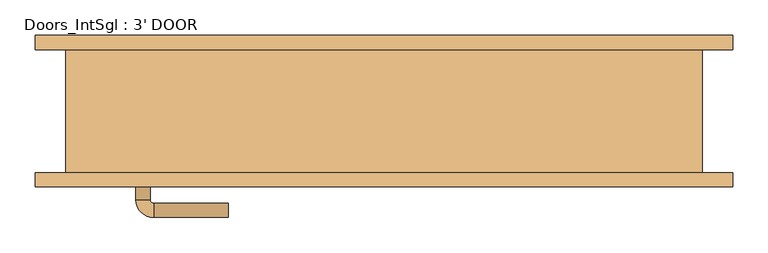
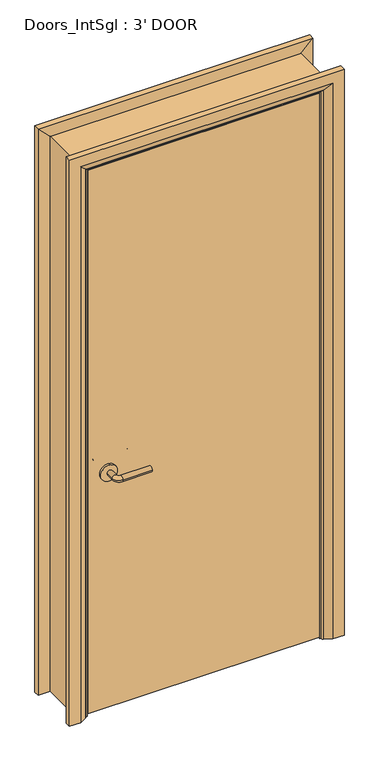
"""IFC4 building model written with IfcOpenShell, lengths in millimetres: door geometry, Doors_IntSgl : 3' DOOR."""

from ifc_helpers import new_model, si_unit, point, frame, frame_2d, origin, place, context, project, spatial, polyline, circle_curve, ellipse_curve, trimmed, segment, composite_curve, outline, extrude, faceted_brep, source, transform, mapped, element, save
from ifc_brep_helpers import plane_surface, cylinder_surface, revolved_surface, advanced_brep


def doors_intsgl_3_door_8261d8fb(model_context):
    return source(origin(), model_context, "Body", "SolidModel", [
        advanced_brep(
        [(-350.2, -40.868, 900.0), (-330.2, -40.868, 900.0), (-350.2, -10.868, 900.0), (-330.2, -10.868, 900.0), (-325.2, -5.868, 900.0), (-325.2, 14.132, 900.0), (-220.2, 14.132, 900.0), (-220.2, -5.868, 900.0)],
        [
            (0, 1, circle_curve(frame((-340.2, -40.868, 900.0), z_axis=(0.0, -1.0, 0.0), x_axis=(1.0, 0.0, 0.0)), 10.0)),
            (1, 0, circle_curve(frame((-340.2, -40.868, 900.0), z_axis=(0.0, -1.0, 0.0), x_axis=(1.0, 0.0, 0.0)), 10.0)),
            (0, 2),
            (2, 3, circle_curve(frame((-340.2, -10.868, 900.0), z_axis=(0.0, -1.0, 0.0), x_axis=(1.0, 0.0, 0.0)), 10.0)),
            (3, 1),
            (3, 2, circle_curve(frame((-340.2, -10.868, 900.0), z_axis=(0.0, -1.0, 0.0), x_axis=(1.0, 0.0, 0.0)), 10.0)),
            (4, 3, circle_curve(frame((-325.2, -10.868, 900.0), z_axis=(0.0, 0.0, 1.0), x_axis=(-1.0, 0.0, 0.0)), 5.0)),
            (2, 5, circle_curve(frame((-325.2, -10.868, 900.0), z_axis=(0.0, 0.0, -1.0), x_axis=(-1.0, 0.0, 0.0)), 25.0)),
            (5, 4, circle_curve(frame((-325.2, 4.132, 900.0), z_axis=(-1.0, 0.0, 0.0), x_axis=(0.0, -1.0, 0.0)), 10.0)),
            (4, 5, circle_curve(frame((-325.2, 4.132, 900.0), z_axis=(-1.0, 0.0, 0.0), x_axis=(0.0, -1.0, 0.0)), 10.0)),
            (6, 7, circle_curve(frame((-220.2, 4.132, 900.0), z_axis=(1.0, 0.0, 0.0), x_axis=(0.0, -1.0, 0.0)), 10.0)),
            (7, 6, circle_curve(frame((-220.2, 4.132, 900.0), z_axis=(1.0, 0.0, 0.0), x_axis=(0.0, -1.0, 0.0)), 10.0)),
            (5, 6),
            (7, 4),
        ],
        [
            plane_surface(frame((-340.2, -40.868, 900.0), z_axis=(0.0, -1.0, 0.0), x_axis=(0.0, 0.0, 1.0))),
            cylinder_surface(frame((-340.2, -40.868, 900.0), z_axis=(0.0, -1.0, 0.0), x_axis=(1.0, 0.0, 0.0)), 10.0),
            revolved_surface(trimmed(ellipse_curve(frame((-340.2, -10.868, 900.0), z_axis=(0.0, -1.0, 0.0), x_axis=(1.0, 0.0, 0.0)), 10.0, 10.0), [point((-350.2, -10.868, 900.0))], [point((-330.2, -10.868, 900.0))], True, "CARTESIAN"), (-325.2, -10.868, 900.0), (0.0, 0.0, -1.0)),
            revolved_surface(trimmed(ellipse_curve(frame((-340.2, -10.868, 900.0), z_axis=(0.0, -1.0, 0.0), x_axis=(1.0, 0.0, 0.0)), 10.0, 10.0), [point((-330.2, -10.868, 900.0))], [point((-350.2, -10.868, 900.0))], True, "CARTESIAN"), (-325.2, -10.868, 900.0), (0.0, 0.0, -1.0)),
            plane_surface(frame((-220.2, 4.132, 900.0), z_axis=(1.0, 0.0, 0.0), x_axis=(0.0, 0.0, 1.0))),
            cylinder_surface(frame((-325.2, 4.132, 900.0), z_axis=(-1.0, 0.0, 0.0), x_axis=(0.0, -1.0, 0.0)), 10.0),
        ],
        [
            (0, [[1, 2]]),
            (1, [[-1, 3, 4, 5]]),
            (1, [[-2, -5, 6, -3]]),
            (2, [[7, -4, 8, 9]]),
            (3, [[-8, -6, -7, 10]]),
            (4, [[11, 12]]),
            (5, [[-9, 13, -12, 14]]),
            (5, [[-10, -14, -11, -13]]),
        ],
    ),
        extrude(outline(composite_curve([segment(trimmed(circle_curve(frame_2d((900.0, -342.7)), 30.0), [point((900.0, -372.7))], [point((900.0, -312.7))], False, "CARTESIAN"), True, "CONTINUOUS"), segment(trimmed(circle_curve(frame_2d((900.0, -342.7)), 30.0), [point((900.0, -312.7))], [point((900.0, -372.7))], False, "CARTESIAN"), True, "CONTINUOUS")], self_intersect=False)), frame((0.0, -48.868, 0.0), z_axis=(0.0, 1.0, 0.0), x_axis=(0.0, 0.0, 1.0)), (0.0, 0.0, 1.0), 8.0),
        advanced_brep(
        [(-350.2, -94.868, 900.0), (-330.2, -94.868, 900.0), (-330.2, -124.868, 900.0), (-350.2, -124.868, 900.0), (-325.2, -129.868, 900.0), (-325.2, -149.868, 900.0), (-220.2, -149.868, 900.0), (-220.2, -129.868, 900.0)],
        [
            (0, 1, circle_curve(frame((-340.2, -94.868, 900.0), z_axis=(0.0, 1.0, 0.0), x_axis=(1.0, 0.0, 0.0)), 10.0)),
            (1, 0, circle_curve(frame((-340.2, -94.868, 900.0), z_axis=(0.0, 1.0, 0.0), x_axis=(1.0, 0.0, 0.0)), 10.0)),
            (1, 2),
            (2, 3, circle_curve(frame((-340.2, -124.868, 900.0), z_axis=(0.0, 1.0, 0.0), x_axis=(1.0, 0.0, 0.0)), 10.0)),
            (3, 0),
            (3, 2, circle_curve(frame((-340.2, -124.868, 900.0), z_axis=(0.0, 1.0, 0.0), x_axis=(1.0, 0.0, 0.0)), 10.0)),
            (4, 5, circle_curve(frame((-325.2, -139.868, 900.0), z_axis=(-1.0, 0.0, 0.0), x_axis=(0.0, 1.0, 0.0)), 10.0)),
            (5, 3, circle_curve(frame((-325.2, -124.868, 900.0), z_axis=(0.0, 0.0, -1.0), x_axis=(-1.0, 0.0, 0.0)), 25.0)),
            (2, 4, circle_curve(frame((-325.2, -124.868, 900.0), z_axis=(0.0, 0.0, 1.0), x_axis=(-1.0, 0.0, 0.0)), 5.0)),
            (5, 4, circle_curve(frame((-325.2, -139.868, 900.0), z_axis=(-1.0, 0.0, 0.0), x_axis=(0.0, 1.0, 0.0)), 10.0)),
            (6, 7, circle_curve(frame((-220.2, -139.868, 900.0), z_axis=(1.0, 0.0, 0.0), x_axis=(0.0, 1.0, 0.0)), 10.0)),
            (7, 6, circle_curve(frame((-220.2, -139.868, 900.0), z_axis=(1.0, 0.0, 0.0), x_axis=(0.0, 1.0, 0.0)), 10.0)),
            (4, 7),
            (6, 5),
        ],
        [
            plane_surface(frame((-340.2, -94.868, 900.0), z_axis=(0.0, 1.0, 0.0), x_axis=(0.0, 0.0, 1.0))),
            cylinder_surface(frame((-340.2, -94.868, 900.0), z_axis=(0.0, 1.0, 0.0), x_axis=(1.0, 0.0, 0.0)), 10.0),
            revolved_surface(trimmed(ellipse_curve(frame((-340.2, -124.868, 900.0), z_axis=(0.0, -1.0, 0.0), x_axis=(1.0, 0.0, 0.0)), 10.0, 10.0), [point((-350.2, -124.868, 900.0))], [point((-330.2, -124.868, 900.0))], True, "CARTESIAN"), (-325.2, -124.868, 900.0), (0.0, 0.0, -1.0)),
            revolved_surface(trimmed(ellipse_curve(frame((-340.2, -124.868, 900.0), z_axis=(0.0, -1.0, 0.0), x_axis=(1.0, 0.0, 0.0)), 10.0, 10.0), [point((-330.2, -124.868, 900.0))], [point((-350.2, -124.868, 900.0))], True, "CARTESIAN"), (-325.2, -124.868, 900.0), (0.0, 0.0, -1.0)),
            plane_surface(frame((-220.2, -139.868, 900.0), z_axis=(1.0, 0.0, 0.0), x_axis=(0.0, 0.0, 1.0))),
            cylinder_surface(frame((-325.2, -139.868, 900.0), z_axis=(-1.0, 0.0, 0.0), x_axis=(0.0, 1.0, 0.0)), 10.0),
        ],
        [
            (0, [[1, 2]]),
            (1, [[3, 4, 5, -2]]),
            (1, [[-5, 6, -3, -1]]),
            (2, [[7, 8, -4, 9]]),
            (3, [[10, -9, -6, -8]]),
            (4, [[11, 12]]),
            (5, [[13, -11, 14, -7]]),
            (5, [[-14, -12, -13, -10]]),
        ],
    ),
        extrude(outline(composite_curve([segment(trimmed(circle_curve(frame_2d((900.0, -342.7)), 30.0), [point((900.0, -372.7))], [point((900.0, -312.7))], False, "CARTESIAN"), True, "CONTINUOUS"), segment(trimmed(circle_curve(frame_2d((900.0, -342.7)), 30.0), [point((900.0, -312.7))], [point((900.0, -372.7))], False, "CARTESIAN"), True, "CONTINUOUS")], self_intersect=False)), frame((0.0, -94.868, 0.0), z_axis=(0.0, 1.0, 0.0), x_axis=(0.0, 0.0, 1.0)), (0.0, 0.0, 1.0), 8.0),
        extrude(outline(polyline([(415.2, -48.868), (415.2, -86.868), (-415.2, -86.868), (-415.2, -48.868), (415.2, -48.868)])), frame((0.0, 0.0, 8.0), z_axis=(0.0, 0.0, 1.0), x_axis=(1.0, 0.0, 0.0)), (0.0, 0.0, 1.0), 2060.0),
        advanced_brep(
        [(492.2, -106.868, 0.0), (452.2, -106.868, 0.0), (426.2, -92.868, 0.0), (422.2, -86.868, 0.0), (492.2, -86.868, 0.0), (492.2, -86.868, 2145.0), (492.2, -106.868, 2145.0), (422.2, -86.868, 2075.0), (-422.2, -86.868, 2075.0), (-422.2, -86.868, 0.0), (-492.2, -86.868, 0.0), (-492.2, -86.868, 2145.0), (426.2, -92.868, 2079.0), (452.2, -106.868, 2105.0), (-492.2, -106.868, 2145.0), (-492.2, -106.868, 0.0), (-452.2, -106.868, 0.0), (-452.2, -106.868, 2105.0), (-426.2, -92.868, 0.0), (-426.2, -92.868, 2079.0)],
        [
            (0, 1),
            (1, 2),
            (2, 3, circle_curve(frame((430.2, -85.868, 0.0), z_axis=(0.0, 0.0, -1.0), x_axis=(1.0, 0.0, 0.0)), 8.0622577)),
            (3, 4),
            (4, 0),
            (4, 5),
            (5, 6),
            (6, 0),
            (3, 7),
            (7, 8),
            (8, 9),
            (9, 10),
            (10, 11),
            (11, 5),
            (2, 12),
            (12, 7, ellipse_curve(frame((430.2, -85.868, 2083.0), z_axis=(0.7071067811865475, 0.0, -0.7071067811865475), x_axis=(-0.7071067811865474, 0.0, -0.7071067811865476)), 11.4017543, 8.0622577)),
            (1, 13),
            (13, 12),
            (6, 14),
            (14, 15),
            (15, 16),
            (16, 17),
            (17, 13),
            (10, 15),
            (14, 11),
            (9, 18, circle_curve(frame((-430.2, -85.868, 0.0), z_axis=(0.0, 0.0, -1.0), x_axis=(-1.0, 0.0, 0.0)), 8.0622577)),
            (18, 16),
            (19, 18),
            (8, 19, ellipse_curve(frame((-430.2, -85.868, 2083.0), z_axis=(-0.7071067811865475, 0.0, -0.7071067811865475), x_axis=(-0.7071067811865474, 0.0, 0.7071067811865476)), 11.4017543, 8.0622577)),
            (19, 17),
            (12, 19),
        ],
        [
            plane_surface(frame((422.2, -86.868, 0.0), z_axis=(0.0, 0.0, -1.0), x_axis=(0.0, 1.0, 0.0))),
            plane_surface(frame((492.2, -106.868, 0.0), z_axis=(1.0, 0.0, 0.0), x_axis=(0.0, 0.0, 1.0))),
            plane_surface(frame((492.2, -86.868, 0.0), z_axis=(0.0, 1.0, 0.0), x_axis=(0.0, 0.0, 1.0))),
            cylinder_surface(frame((430.2, -85.868, 0.0), z_axis=(0.0, 0.0, -1.0), x_axis=(1.0, 0.0, 0.0)), 8.0622577),
            plane_surface(frame((426.2, -92.868, 0.0), z_axis=(-0.4740998230350126, -0.880471099922178, 0.0), x_axis=(0.0, 0.0, 1.0))),
            plane_surface(frame((452.2, -106.868, 0.0), z_axis=(0.0, -1.0, 0.0), x_axis=(0.0, 0.0, 1.0))),
            plane_surface(frame((-492.2, -106.868, 2145.0), z_axis=(-1.0, 0.0, 0.0), x_axis=(0.0, 0.0, -1.0))),
            plane_surface(frame((-422.2, -86.868, 0.0), z_axis=(0.0, 0.0, -1.0), x_axis=(0.0, 1.0, 0.0))),
            cylinder_surface(frame((-430.2, -85.868, 2075.0), z_axis=(0.0, 0.0, 1.0), x_axis=(-1.0, 0.0, 0.0)), 8.0622577),
            plane_surface(frame((-426.2, -92.868, 2079.0), z_axis=(0.47409982303501824, -0.8804710999221749, 0.0), x_axis=(0.0, 0.0, -1.0))),
            plane_surface(frame((492.2, -106.868, 2145.0), z_axis=(0.0, 0.0, 1.0), x_axis=(-1.0, 0.0, 0.0))),
            cylinder_surface(frame((422.2, -85.868, 2083.0), z_axis=(1.0, 0.0, 0.0), x_axis=(0.0, 0.0, 1.0)), 8.0622577),
            plane_surface(frame((426.2, -92.868, 2079.0), z_axis=(0.0, -0.8804710999221764, -0.4740998230350154), x_axis=(-1.0, 0.0, 0.0))),
        ],
        [
            (0, [[1, 2, 3, 4, 5]]),
            (1, [[6, 7, 8, -5]]),
            (2, [[9, 10, 11, 12, 13, 14, -6, -4]]),
            (3, [[15, 16, -9, -3]]),
            (4, [[17, 18, -15, -2]]),
            (5, [[-8, 19, 20, 21, 22, 23, -17, -1]]),
            (6, [[-13, 24, -20, 25]]),
            (7, [[-24, -12, 26, 27, -21]]),
            (8, [[28, -26, -11, 29]]),
            (9, [[-22, -27, -28, 30]]),
            (10, [[-14, -25, -19, -7]]),
            (11, [[31, -29, -10, -16]]),
            (12, [[-23, -30, -31, -18]]),
        ],
    ),
        extrude(outline(polyline([(0.0, -398.2), (2051.0, -398.2), (2051.0, 398.2), (0.0, 398.2), (0.0, 417.2), (2070.0, 417.2), (2070.0, -417.2), (0.0, -417.2), (0.0, -398.2)])), frame((0.0, -46.868, 0.0), z_axis=(0.0, 1.0, 0.0), x_axis=(0.0, 0.0, 1.0)), (0.0, 0.0, 1.0), 32.0),
        advanced_brep(
        [(-492.2, 106.868, 0.0), (-452.2, 106.868, 0.0), (-426.2, 92.868, 0.0), (-422.2, 86.868, 0.0), (-492.2, 86.868, 0.0), (-492.2, 86.868, 2145.0), (-492.2, 106.868, 2145.0), (-422.2, 86.868, 2075.0), (-426.2, 92.868, 2079.0), (-452.2, 106.868, 2105.0), (492.2, 106.868, 0.0), (492.2, 86.868, 0.0), (422.2, 86.868, 0.0), (426.2, 92.868, 0.0), (452.2, 106.868, 0.0), (492.2, 106.868, 2145.0), (452.2, 106.868, 2105.0), (426.2, 92.868, 2079.0), (422.2, 86.868, 2075.0), (492.2, 86.868, 2145.0)],
        [
            (0, 1),
            (1, 2),
            (2, 3, circle_curve(frame((-430.2, 85.868, 0.0), z_axis=(0.0, 0.0, -1.0), x_axis=(-1.0, 0.0, 0.0)), 8.0622577)),
            (3, 4),
            (4, 0),
            (4, 5),
            (5, 6),
            (6, 0),
            (3, 7),
            (7, 5),
            (2, 8),
            (8, 7, ellipse_curve(frame((-430.2, 85.868, 2083.0), z_axis=(-0.7071067811865475, 0.0, -0.7071067811865475), x_axis=(0.7071067811865474, 0.0, -0.7071067811865476)), 11.4017543, 8.0622577)),
            (1, 9),
            (9, 8),
            (6, 9),
            (10, 11),
            (11, 12),
            (12, 13, circle_curve(frame((430.2, 85.868, 0.0), z_axis=(0.0, 0.0, -1.0), x_axis=(1.0, 0.0, 0.0)), 8.0622577)),
            (13, 14),
            (14, 10),
            (15, 10),
            (14, 16),
            (16, 15),
            (13, 17),
            (17, 16),
            (12, 18),
            (18, 17, ellipse_curve(frame((430.2, 85.868, 2083.0), z_axis=(0.7071067811865475, 0.0, -0.7071067811865475), x_axis=(0.7071067811865474, 0.0, 0.7071067811865476)), 11.4017543, 8.0622577)),
            (11, 19),
            (19, 18),
            (15, 19),
            (5, 19),
            (15, 6),
            (7, 18),
            (8, 17),
            (9, 16),
        ],
        [
            plane_surface(frame((-422.2, 159.6690989, 0.0), z_axis=(0.0, 0.0, -1.0), x_axis=(1.0, 0.0, 0.0))),
            plane_surface(frame((-492.2, 106.868, 0.0), z_axis=(-1.0, 0.0, 0.0), x_axis=(0.0, 0.0, 1.0))),
            plane_surface(frame((-492.2, 86.868, 0.0), z_axis=(0.0, -1.0, 0.0), x_axis=(0.0, 0.0, 1.0))),
            cylinder_surface(frame((-430.2, 85.868, 0.0), z_axis=(0.0, 0.0, -1.0), x_axis=(-1.0, 0.0, 0.0)), 8.0622577),
            plane_surface(frame((-426.2, 92.868, 0.0), z_axis=(0.4740998230350183, 0.8804710999221749, 0.0), x_axis=(0.0, 0.0, 1.0))),
            plane_surface(frame((-452.2, 106.868, 0.0), z_axis=(0.0, 1.0, 0.0), x_axis=(0.0, 0.0, 1.0))),
            plane_surface(frame((422.2, 159.6690989, 0.0), z_axis=(0.0, 0.0, -1.0), x_axis=(-1.0, 0.0, 0.0))),
            plane_surface(frame((452.2, 106.868, 2105.0), z_axis=(0.0, 1.0, 0.0), x_axis=(0.0, 0.0, -1.0))),
            plane_surface(frame((426.2, 92.868, 2079.0), z_axis=(-0.4740998230350183, 0.8804710999221749, 0.0), x_axis=(0.0, 0.0, -1.0))),
            cylinder_surface(frame((430.2, 85.868, 2075.0), z_axis=(0.0, 0.0, 1.0), x_axis=(1.0, 0.0, 0.0)), 8.0622577),
            plane_surface(frame((492.2, 86.868, 2145.0), z_axis=(0.0, -1.0, 0.0), x_axis=(0.0, 0.0, -1.0))),
            plane_surface(frame((492.2, 106.868, 2145.0), z_axis=(1.0, 0.0, 0.0), x_axis=(0.0, 0.0, -1.0))),
            plane_surface(frame((-492.2, 106.868, 2145.0), z_axis=(0.0, 0.0, 1.0), x_axis=(1.0, 0.0, 0.0))),
            plane_surface(frame((-492.2, 86.868, 2145.0), z_axis=(0.0, -1.0, 0.0), x_axis=(1.0, 0.0, 0.0))),
            cylinder_surface(frame((-422.2, 85.868, 2083.0), z_axis=(-1.0, 0.0, 0.0), x_axis=(0.0, 0.0, 1.0)), 8.0622577),
            plane_surface(frame((-426.2, 92.868, 2079.0), z_axis=(0.0, 0.8804710999221749, -0.4740998230350183), x_axis=(1.0, 0.0, 0.0))),
            plane_surface(frame((-452.2, 106.868, 2105.0), z_axis=(0.0, 1.0, 0.0), x_axis=(1.0, 0.0, 0.0))),
        ],
        [
            (0, [[1, 2, 3, 4, 5]]),
            (1, [[6, 7, 8, -5]]),
            (2, [[9, 10, -6, -4]]),
            (3, [[11, 12, -9, -3]]),
            (4, [[13, 14, -11, -2]]),
            (5, [[-8, 15, -13, -1]]),
            (6, [[16, 17, 18, 19, 20]]),
            (7, [[21, -20, 22, 23]]),
            (8, [[-22, -19, 24, 25]]),
            (9, [[-24, -18, 26, 27]]),
            (10, [[-26, -17, 28, 29]]),
            (11, [[-28, -16, -21, 30]]),
            (12, [[31, -30, 32, -7]]),
            (13, [[33, -29, -31, -10]]),
            (14, [[34, -27, -33, -12]]),
            (15, [[35, -25, -34, -14]]),
            (16, [[-32, -23, -35, -15]]),
        ],
    ),
        faceted_brep([(-417.2, -86.868, 0.0), (-449.2, -86.868, 0.0), (-449.2, 86.868, 0.0), (-417.2, 86.868, 0.0), (-417.2, 86.868, 2070.0), (-417.2, -86.868, 2070.0), (-449.2, 86.868, 2102.0), (-449.2, -86.868, 2102.0), (417.2, -86.868, 0.0), (417.2, 86.868, 0.0), (449.2, 86.868, 0.0), (449.2, -86.868, 0.0), (417.2, -86.868, 2070.0), (449.2, -86.868, 2102.0), (449.2, 86.868, 2102.0), (417.2, 86.868, 2070.0)], [[[0, 1, 2, 3]], [[3, 4, 5, 0]], [[2, 6, 4, 3]], [[1, 7, 6, 2]], [[0, 5, 7, 1]], [[8, 9, 10, 11]], [[12, 8, 11, 13]], [[13, 11, 10, 14]], [[14, 10, 9, 15]], [[15, 9, 8, 12]], [[4, 15, 12, 5]], [[6, 14, 15, 4]], [[7, 13, 14, 6]], [[5, 12, 13, 7]]]),
    ])


if __name__ == "__main__":
    model = new_model("IFC4")
    model_context = context("Model", 3, world=origin())
    ifc_project = project(units=[si_unit("LENGTHUNIT", "METRE", prefix="MILLI")], contexts=[model_context])
    site = spatial("IfcSite", under=ifc_project)
    building = spatial("IfcBuilding", under=site)
    placement = place(None, origin())
    doors_intsgl_3_door_shape = doors_intsgl_3_door_8261d8fb(model_context)
    element("IfcDoor", 1, ObjectType="Doors_IntSgl : 3' DOOR", at=placement, inside=building, context=model_context, shape_type="MappedRepresentation", body=[
        mapped(doors_intsgl_3_door_shape, transform((0.0, 0.0, 0.0), x_axis=(1.0, 0.0, 0.0), y_axis=(0.0, 1.0, 0.0), z_axis=(0.0, 0.0, 1.0))),
    ])
    save(model, "model.ifc")

# Revit data of these elements
# Type "Doors_IntSgl : 3' DOOR"
#   Type Mark = "46"
#   Type Comments = "Internal Single"
#   Operation = "SingleSwingRight"
#   Manufacturer = "Revit"
#   Keynote = "L20"
#   Description = "Internal Single Door"
#   Analytic Construction = "Metal"
#   UnderCut = 0.026247 ft
#   Tolerance = 0.006562 ft
#   Thickness = 0.124672 ft
#   Thermal Resistance (R) = 0.270117 (m²·K)/W
#   Structural Tolerance = 0.026247 ft
#   StopDepth = 0.104987 ft
#   Stop Thickness = 0.062336 ft
#   Rough Width = 3.0 ft
#   Rough Height = 6.922572 ft
#   Height to Top Lock Rail = 3.28084 ft
#   Heat Transfer Coefficient (U) = 3.7021 W/(m²·K)
#   Handle Z Distance = 2.952756 ft
#   Handle X Distance = 0.246063 ft
#   Frame Thickness = 0.104987 ft
#   Door Panel Width = 2.724409 ft
#   Door Panel Thickness = 0.124672 ft
#   Door Panel Offset = 0.0 ft
#   Height = 6.922572 ft
#   Width = 3.0 ft
#   Door Panel Height = 6.75853 ft
#   Architrave Setback = 0.016404 ft
#   Vis - Ironmongery = yes
#   Material Ironmongery = Door - Handle
#   Material Frame = Door - Frame/Mullion (1)
#   Material Door = Door - Panel
#   Material Architrave = Door - Architrave
#   Visual Light Transmittance = 0
#   Solar Heat Gain Coefficient = 0
#   Function = (empty or 0)
#   Wall Closure = (empty or 0)
# Element 1 (IfcDoor, "Doors_IntSgl : 3' DOOR")
#   Materials on its faces: "Door - Architrave", "Door - Handle", "Door - Frame/Mullion (1)", "Door - Panel"
# Materials
#   "Door - Handle": colour RGB 0 0 0, transparency 0, Keynote = "P21", Cost = 0
#   "Door - Frame/Mullion (1)": class "Wood", colour RGB 212 179 113, transparency 0, Keynote = "L20", Cost = 0
#   "Door - Panel": class "Wood", colour RGB 210 159 95, transparency 0, Keynote = "L20", Cost = 0
#   "Door - Architrave": class "Wood", colour RGB 154 90 5, transparency 0, Keynote = "P20", Cost = 0
